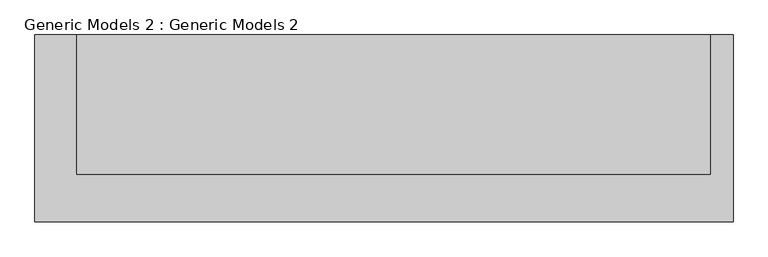
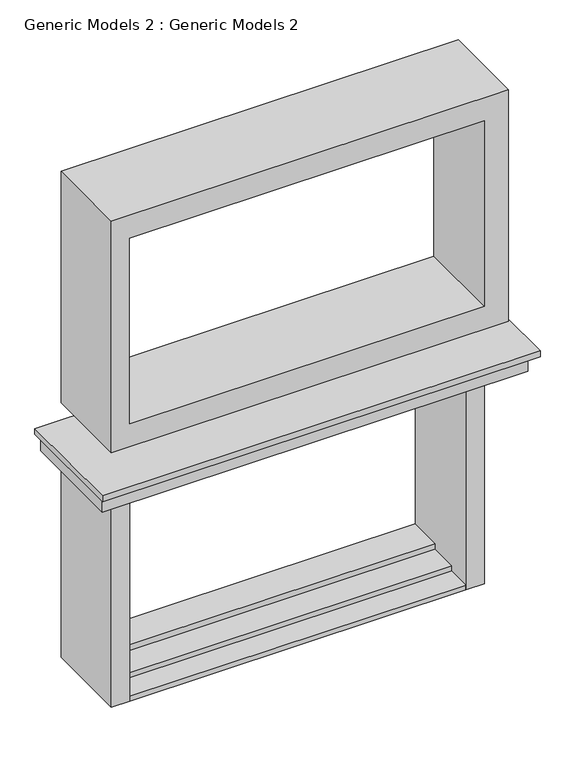
"""IFC4 building model written with IfcOpenShell, lengths in millimetres: proxy geometry, Generic Models 2 : Generic Models 2."""

from ifc_helpers import new_model, si_unit, frame, origin, origin_with_axes, place, context, project, spatial, polyline, outline, extrude, source, transform, mapped, element, save


def generic_models_2_generic_models_2_e7d0f1f0(model_context):
    return source(origin(), model_context, "Body", "SweptSolid", [
        extrude(outline(polyline([(3352.8, -19189.1403308), (3352.8, -14236.1403308), (6400.8, -14236.1403308), (6400.8, -19189.1403308), (3352.8, -19189.1403308)]), holes=[polyline([(6096.0, -14540.9403308), (3652.758733, -14540.9403308), (3652.758733, -18960.5403308), (6096.0, -18960.5403308), (6096.0, -14540.9403308)])]), frame((0.0, -14443.349314, 0.0), z_axis=(0.0, 1.0, 0.0), x_axis=(0.0, 0.0, 1.0)), (0.0, 0.0, 1.0), 1087.9974402),
        extrude(outline(polyline([(-14058.3403308, -14816.4459495), (-19514.6595652, -14816.4459495), (-19514.6595652, -13355.3518738), (-14058.3403308, -13355.3518738), (-14058.3403308, -14816.4459495)])), frame((0.0, 0.0, 3048.0), z_axis=(0.0, 0.0, 1.0), x_axis=(1.0, 0.0, 0.0)), (0.0, 0.0, 1.0), 76.2),
        extrude(outline(polyline([(-14139.3472533, -14686.8687396), (-19443.1403308, -14686.8687396), (-19443.1403308, -13355.3518738), (-14139.3472533, -13355.3518738), (-14139.3472533, -14686.8687396)])), frame((0.0, 0.0, 2806.8529627), z_axis=(0.0, 0.0, 1.0), x_axis=(1.0, 0.0, 0.0)), (0.0, 0.0, 1.0), 241.1470373),
        extrude(outline(polyline([(-19189.1403308, -14443.349314), (-19189.1403308, -13355.3518738), (-18960.5403308, -13355.3518738), (-18960.5403308, -14443.349314), (-19189.1403308, -14443.349314)])), origin_with_axes(), (0.0, 0.0, 1.0), 2858.1133382),
        extrude(outline(polyline([(-14540.9403308, -13355.3518738), (-14540.9403308, -14443.349314), (-14769.5403308, -14443.349314), (-14769.5403308, -13355.3518738), (-14540.9403308, -13355.3518738)])), origin_with_axes(), (0.0, 0.0, 1.0), 2858.1133382),
        extrude(outline(polyline([(-14769.5403308, -14443.349314), (-18960.5403308, -14443.349314), (-18960.5403308, -14138.549314), (-14769.5403308, -14138.549314), (-14769.5403308, -14443.349314)])), origin_with_axes(), (0.0, 0.0, 1.0), 63.1359864),
        extrude(outline(polyline([(-14769.5403308, -14138.549314), (-18960.5403308, -14138.549314), (-18960.5403308, -13780.4379006), (-14769.5403308, -13780.4379006), (-14769.5403308, -14138.549314)])), origin_with_axes(), (0.0, 0.0, 1.0), 133.0827065),
        extrude(outline(polyline([(-14769.5403308, -13780.4379006), (-18960.5403308, -13780.4379006), (-18960.5403308, -13355.3518738), (-14769.5403308, -13355.3518738), (-14769.5403308, -13780.4379006)])), origin_with_axes(), (0.0, 0.0, 1.0), 207.4335771),
    ])


if __name__ == "__main__":
    model = new_model("IFC4")
    model_context = context("Model", 3, world=origin())
    ifc_project = project(units=[si_unit("LENGTHUNIT", "METRE", prefix="MILLI")], contexts=[model_context])
    site = spatial("IfcSite", under=ifc_project)
    building = spatial("IfcBuilding", under=site)
    placement = place(None, origin())
    generic_models_2_generic_models_2_shape = generic_models_2_generic_models_2_e7d0f1f0(model_context)
    element("IfcBuildingElementProxy", 1, Name="Generic Models 2 : Generic Models 2", ObjectType="Generic Models 2 : Generic Models 2", at=placement, inside=building, context=model_context, shape_type="MappedRepresentation", body=[
        mapped(generic_models_2_generic_models_2_shape, transform((0.0, 0.0, 0.0), x_axis=(1.0, 0.0, 0.0), y_axis=(0.0, 1.0, 0.0), z_axis=(0.0, 0.0, 1.0))),
    ])
    save(model, "model.ifc")
